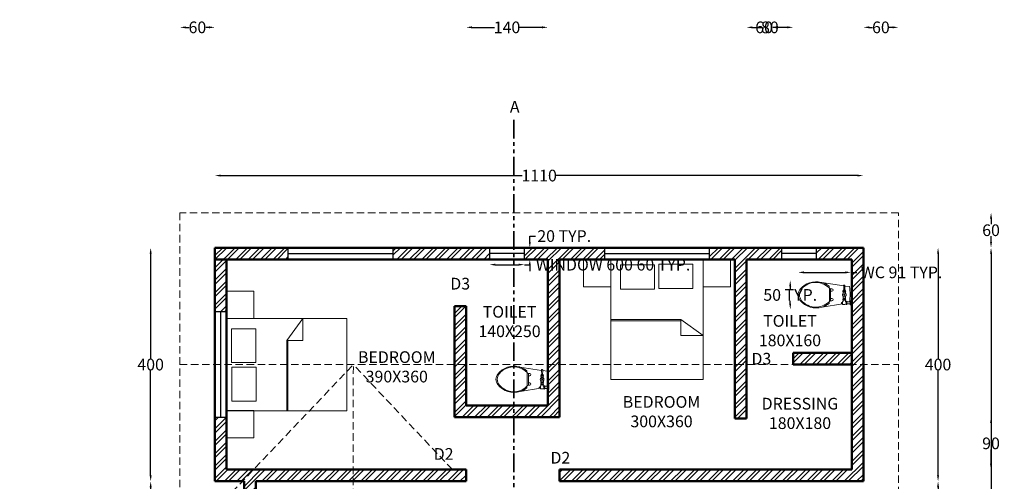
# Model space of a CAD drawing. Units: centimetres. Extents: x 10444 to 13814, y 8288 to 11191.
# Tile 9 of 9: x 12129 to 13814, y 10401 to 11191. Entities that reach past the tile are written whole.
import ezdxf

# ---------------------------------------------------------------- set-up
doc = ezdxf.new("R2010")
doc.units = ezdxf.units.CM
doc.header["$MEASUREMENT"] = 0
doc.linetypes.add('DASHED', pattern=[19.05, 12.7, -6.35])
doc.linetypes.add('PHANTOM', pattern=[63.5, 31.75, -6.35, 6.35, -6.35, 6.35, -6.35])
for name, color, linetype, lineweight in [('A-ANNO-DIMS', 2, 'Continuous', 18), ('A-ANNO-SYMB', 7, 'Continuous', 25), ('A-ANNO-SYMB-SECT', 1, 'PHANTOM', 35), ('A-ANNO-TEXT', 7, 'Continuous', 25), ('A-AREA-IDEN', 3, 'Continuous', 25), ('A-FLOR-FIXT', 9, 'Continuous', 18), ('A-FURN', 8, 'Continuous', 18), ('A-GLAZ', 4, 'Continuous', 25), ('A-ROOF-OVHD', 6, 'DASHED', 18), ('A-WALL', 7, 'Continuous', 50), ('A-WALL-PATT', 8, 'Continuous', 13)]:
    doc.layers.add(name, color=color, linetype=linetype, lineweight=lineweight)
doc.styles.get("Standard").update_dxf_attribs({"font": 'arial.ttf'})
doc.dimstyles.get("Standard").update_dxf_attribs({"dimtxt": 20, "dimasz": 10, "dimexe": 0.18, "dimexo": 0.0625, "dimgap": 0.09, "dimtad": 0, "dimtih": 1, "dimtoh": 1, "dimdec": 0, "dimzin": 0, "dimdsep": 46, "dimtxsty": 'Standard', "dimcen": 0.09, "dimse1": 1, "dimse2": 1, "dimadec": 0, "dimazin": 0, "dimtfac": 1, "dimtdec": 0, "dimtofl": 0, "dimtmove": 0, "dimatfit": 3, "dimfxl": 1, "dimtolj": 1, "dimtzin": 0, "dimarcsym": 0})

# ---------------------------------------------------------------- blocks, each defined once
blk = doc.blocks.new('BED')
for p, q in [((1734.1, 2886.7), (1849.5, 2886.7)), ((1849.5, 2886.7), (1886.1, 2860.2)), ((1886.1, 2860.2), (1849.5, 2886.7)), ((1849.5, 2886.7), (1849.5, 2860.2)), ((1734.1, 2884.7), (1849.5, 2884.7)), ((1849.5, 2860.2), (1886.1, 2860.2))]:
    blk.add_line(p, q)
for points in [[(1734.1, 2787.7), (1886.1, 2787.7), (1886.1, 2985.7), (1734.1, 2985.7)], [(1750, 2936.8), (1805.9, 2936.8), (1805.9, 2977), (1750, 2977)], [(1813.2, 2937.8), (1869.1, 2937.8), (1869.1, 2977.9), (1813.2, 2977.9)]]:
    blk.add_lwpolyline(points, close=True)
blk = doc.blocks.new('TOILETY')
for p, q in [((2296.2, 1053), (2296.2, 1053.3)), ((2296.6, 1052.5), (2297, 1052.5)), ((2297, 1052.5), (2297.7, 1052.5)), ((2297.7, 1052.6), (2297.7, 1052.5)), ((2297.7, 1052.5), (2297.7, 1050.2)), ((2297.7, 1052.5), (2297.7, 1052.5)), ((2303.2, 1052), (2303.2, 1050.7)), ((2307.3, 1052.6), (2307.3, 1052.5)), ((2307.3, 1052.5), (2307.3, 1052.5)), ((2307.3, 1052.5), (2307.3, 1050.2)), ((2297.7, 1050.2), (2297.7, 1050.2)), ((2307.3, 1050.2), (2307.3, 1050.2)), ((2296.5, 1036.2), (2297.2, 1037.4)), ((2297.2, 1037.4), (2297.2, 1038.7)), ((2299.5, 1037.4), (2297.2, 1037.4)), ((2299.5, 1038.7), (2299.5, 1037.4)), ((2303.2, 1037.4), (2299.5, 1037.4)), ((2303.2, 1037.4), (2306.9, 1037.4)), ((2306.9, 1038.7), (2306.9, 1037.4)), ((2306.9, 1037.4), (2309.3, 1037.4)), ((2309.3, 1037.4), (2309.3, 1038.7)), ((2309.9, 1036.2), (2309.3, 1037.4))]:
    blk.add_line(p, q)
for points in [[(2293.8, 1057.3), (2293.3, 1057.3, -0.293225), (2292.6, 1058.4), (2295, 1058.4), (2297.2, 1058.4, -0.293225), (2296.5, 1057.3), (2296, 1057.3)], [(2293.8, 1054.1), (2293.6, 1054.1, 0.913215), (2293.6, 1053.3)], [(2295, 1057.3), (2293.8, 1057.3, -0.293225)], [(2294.9, 1054.1), (2293.8, 1054.1, 0.913215)], [(2294.9, 1054.1), (2296, 1054.1, -0.913215)], [(2295, 1057.3), (2296, 1057.3, 0.335115)], [(2296, 1056.9, -0.066772), (2311.6, 1056.7, -11.173493)], [(2296, 1054.1), (2296.2, 1054.1, -0.913215), (2296.2, 1053.3), (2296.1, 1053.3)], [(2297.8, 1052.7, 0.071269), (2297.8, 1052.5, 0.085783), (2297.9, 1052.4, 0.10607), (2298, 1052.2, 0.126822), (2298.2, 1052.2, 0.126822), (2298.4, 1052.2, 0.10607), (2298.5, 1052.4, 0.085783), (2298.6, 1052.5, 0.071269), (2298.6, 1052.7, 0.075445)], [(2298.7, 1052.6, 0.236068), (2298.8, 1052.5), (2299.8, 1052.5, 0.868488)], [(2306.3, 1052.6, -0.236068), (2306.2, 1052.5), (2304.8, 1052.5, -0.947474)], [(2307.2, 1052.7, -0.071269), (2307.2, 1052.5, -0.085783), (2307.1, 1052.4, -0.10607), (2307, 1052.2, -0.126822), (2306.8, 1052.2, -0.126822), (2306.6, 1052.2, -0.10607), (2306.5, 1052.4, -0.085783), (2306.4, 1052.5, -0.071269), (2306.4, 1052.7, -0.075445)], [(2307.3, 1052.5, 0.414214), (2307.4, 1052.4), (2307.9, 1052.5, -0.274044), (2308, 1052.4), (2308, 1051.9)], [(2308, 1051.9, 0.386607), (2308.3, 1051.8), (2312.2, 1052, -0.016038)], [(2312.2, 1052), (2311.6, 1056.7, 0.064477)], [(2312.2, 1052), (2312.7, 1052, -0.016603), (2312.7, 1052, -1.33807)], [(2312.7, 1052, -0.398884), (2313.2, 1051.6), (2313.2, 1051.4)], [(2312.7, 1050.7, 0.398884), (2313.2, 1051.2), (2313.2, 1051.4)], [(2290.7, 1028.8), (2294, 1049.6, -0.075157)], [(2297.8, 1050.1, -0.056795), (2297.8, 1050.3, -0.085783), (2297.9, 1050.5, -0.10607), (2298, 1050.6, -0.126822), (2298.2, 1050.6, -0.126822), (2298.4, 1050.6, -0.10607), (2298.5, 1050.5, -0.085783), (2298.6, 1050.3, -0.056795), (2298.6, 1050.1, -0.075445)], [(2298.7, 1050.2, -0.236068), (2298.8, 1050.3), (2299.8, 1050.3, -0.868488)], [(2306.3, 1050.2, 0.236068), (2306.2, 1050.3), (2304.8, 1050.3, 0.947474)], [(2307.2, 1050.1, 0.056795), (2307.2, 1050.3, 0.085783), (2307.1, 1050.5, 0.10607), (2307, 1050.6, 0.126822), (2306.8, 1050.6, 0.126822), (2306.6, 1050.6, 0.10607), (2306.5, 1050.5, 0.085783), (2306.4, 1050.3, 0.056795), (2306.4, 1050.1, 0.075445)], [(2307.3, 1050.2, -0.414214), (2307.4, 1050.3), (2307.9, 1050.3, 0.274044), (2308, 1050.3), (2308, 1050.8)], [(2308, 1050.8, -0.386607), (2308.3, 1051), (2312.4, 1050.8, 0.016063)], [(2312.4, 1050.8), (2312.7, 1050.7, 0.016603), (2312.7, 1050.7, 1.33807)], [(2315.8, 1028.5), (2312.4, 1050.8, 0.07524)], [(2296, 1035.7, 0.434217), (2297.2, 1007.6, 0.182634), (2303.2, 1005.4, 2.693815)], [(2294.4, 1035.7, 0.094048), (2290.7, 1028.8, 0.16845)], [(2296, 1035.7), (2294.4, 1035.7, 0.416606)], [(2296.5, 1036.2, 0.008985), (2296, 1035.7, 0.182634)], [(2303.2, 1036.2), (2296.5, 1036.2, 0.008985)], [(2303.2, 1036.2), (2309.9, 1036.2, -0.444938)], [(2310.4, 1035.7, -0.434217), (2309.3, 1007.6, -0.182634), (2303.2, 1005.4, -2.693815)], [(2309.9, 1036.2, -0.008985), (2310.4, 1035.7, -0.182634)], [(2310.4, 1035.7), (2312, 1035.7, -0.416606)], [(2312, 1035.7, -0.105447), (2316, 1027.8, -0.16845)], [(2290.7, 1028.8, 0.310397), (2297.8, 1005.9, 0.16845), (2303.2, 1004, 2.883082)], [(2316, 1027.8, -0.298065), (2308.6, 1005.9, -0.16845), (2303.2, 1004, -2.883082)], [(2316, 1027.8, 0.006132), (2315.8, 1028.5, 0.069947)]]:
    blk.add_lwpolyline(points, format="xyb")
for points in [[(2293.6, 1053.3), (2293.6, 1052.5), (2293.3, 1051.8), (2293.3, 1049.8)], [(2296.2, 1053.3), (2293.6, 1053.3)], [(2293.8, 1054.1), (2293.8, 1057.3)], [(2296, 1056.9), (2296, 1057.3)], [(2296, 1054.1), (2296, 1056.9)], [(2298.7, 1050.2), (2298.7, 1052.6)], [(2299.8, 1052.5), (2299.8, 1052.7), (2301.9, 1052.7)], [(2299.8, 1052.5), (2299.8, 1050.3)], [(2306.3, 1050.2), (2306.3, 1052.6)], [(2308, 1051.9), (2308, 1051.4)], [(2308, 1050.8), (2308, 1051.4)], [(2294, 1049.6), (2293.4, 1049.6), (2293.3, 1049.8)], [(2294.2, 1049.6), (2294, 1049.6)], [(2294.2, 1049.5), (2294.2, 1049.6)], [(2295.4, 1049.6), (2294.2, 1049.6)], [(2294.2, 1049.5), (2294.2, 1049.5)], [(2294.2, 1049.5), (2295.4, 1049.5)], [(2294.3, 1048.9), (2294.2, 1048.9), (2294.2, 1049.5)], [(2294.2, 1049.5), (2294.5, 1049.4), (2294.8, 1049.5), (2295.2, 1049.4), (2295.4, 1049.5)], [(2294.2, 1048.9), (2294.5, 1049), (2294.8, 1048.9), (2295.2, 1049), (2295.4, 1048.9)], [(2294.3, 1048.9), (2294.3, 1048.5), (2294.6, 1048.5)], [(2295.3, 1048.9), (2294.3, 1048.9)], [(2294.5, 1049), (2294.5, 1049.4)], [(2294.6, 1048.5), (2295.3, 1048.5), (2295.3, 1048.9)], [(2295.2, 1049), (2295.2, 1049.4)], [(2295.4, 1049.5), (2295.4, 1049.5), (2295.4, 1048.9), (2295.3, 1048.9)], [(2296.3, 1049.8), (2296.3, 1049.6), (2295.4, 1049.6)], [(2295.4, 1049.5), (2295.4, 1049.6)], [(2296.3, 1049.8), (2296.6, 1050.2)], [(2296.6, 1050.2), (2297.7, 1050.2)], [(2299.8, 1050.3), (2299.8, 1050.1), (2301.8, 1050.1)]]:
    blk.add_lwpolyline(points)
for points in [[(2294.9, 1053.3, 0.06206), (2295.2, 1053.4, 0.075298), (2295.4, 1053.4, 0.107049), (2295.5, 1053.6, 0.150029), (2295.5, 1053.7, 0.150029), (2295.5, 1053.8, 0.107049), (2295.4, 1054, 0.075298), (2295.2, 1054.1, 0.06206), (2294.9, 1054.1, 0.06206), (2294.7, 1054.1, 0.075298), (2294.5, 1054, 0.107049), (2294.3, 1053.8, 0.150029), (2294.3, 1053.7, 0.150029), (2294.3, 1053.6, 0.107049), (2294.5, 1053.4, 0.075298), (2294.7, 1053.4, 0.06206)], [(2298.6, 1051.4, -0.075445), (2298.6, 1051.2, -0.085783), (2298.5, 1051, -0.10607), (2298.4, 1050.8, -0.126822), (2298.2, 1050.8, -0.126822), (2298, 1050.8, -0.10607), (2297.9, 1051, -0.085783), (2297.8, 1051.2, -0.075445), (2297.8, 1051.4, -0.075445), (2297.8, 1051.6, -0.085783), (2297.9, 1051.8, -0.10607), (2298, 1051.9, -0.126822), (2298.2, 1051.9, -0.126822), (2298.4, 1051.9, -0.10607), (2298.5, 1051.8, -0.085783), (2298.6, 1051.6, -0.075445)], [(2306.4, 1051.4, 0.075445), (2306.4, 1051.2, 0.085783), (2306.5, 1051, 0.10607), (2306.6, 1050.8, 0.126822), (2306.8, 1050.8, 0.126822), (2307, 1050.8, 0.10607), (2307.1, 1051, 0.085783), (2307.2, 1051.2, 0.075445), (2307.2, 1051.4, 0.075445), (2307.2, 1051.6, 0.085783), (2307.1, 1051.8, 0.10607), (2307, 1051.9, 0.126822), (2306.8, 1051.9, 0.126822), (2306.6, 1051.9, 0.10607), (2306.5, 1051.8, 0.085783), (2306.4, 1051.6, 0.075445)]]:
    blk.add_lwpolyline(points, format="xyb", close=True)
blk.add_lwpolyline([(2303.2, 1052), (2302.6, 1051.7), (2302.6, 1051), (2303.2, 1050.7), (2303.8, 1051), (2303.8, 1051.7)], close=True)
blk.add_circle((2303.2, 1051.4), 1.91)
for centre, radius, start, end in [((2293.7, 1053.7), 0.391, 275.1944, 84.8056), ((2296.1, 1053.7), 0.391, 95.1944, 264.8056), ((2296.7, 1053), 0.527, 178.4608, 258.8588), ((2298.2, 1052.3), 0.551, 33.3985, 146.6015), ((2306.8, 1052.3), 0.551, 33.3985, 146.6015), ((2298.2, 1050.5), 0.551, 213.3985, 326.6015), ((2306.8, 1050.5), 0.551, 213.3985, 326.6015), ((2298.3, 1038.7), 1.16, 0, 180), ((2308.1, 1038.7), 1.16, 0, 180)]:
    blk.add_arc(centre, radius, start, end)
blk = doc.blocks.new('*D15')
at = {"layer": 'A-ANNO-DIMS', "color": 0, "lineweight": -2, "transparency": 16777216}
for p, q in [((12473.1, 10924.2), (12989.1, 10924.2)), ((13563.1, 10924.2), (13047.1, 10924.2))]:
    blk.add_line(p, q, dxfattribs=at)
at = {"layer": 'A-ANNO-DIMS', "color": 0, "transparency": 16777216}
for points in [[(12473.1, 10925.8), (12473.1, 10922.5), (12463.1, 10924.2)], [(13563.1, 10925.8), (13563.1, 10922.5), (13573.1, 10924.2)]]:
    blk.add_solid(points, dxfattribs=at)
at = {"layer": 'Defpoints', "color": 0, "transparency": 16777216}
for p in [(13573.1, 10924.2), (12463.1, 10800.6), (13573.1, 10800.6)]:
    blk.add_point(p, dxfattribs=at)
at = {"layer": 'A-ANNO-DIMS', "color": 0, "transparency": 16777216, "insert": (13018.1, 10924.2), "char_height": 20, "attachment_point": 5}
blk.add_mtext('\\A1;1110', dxfattribs=at)
blk = doc.blocks.new('*D16')
at = {"layer": 'A-ANNO-DIMS', "color": 0, "lineweight": -2, "transparency": 16777216}
for p, q in [((12353.1, 10790.6), (12353.1, 10610.9)), ((12353.1, 10410.6), (12353.1, 10590.3))]:
    blk.add_line(p, q, dxfattribs=at)
at = {"layer": 'A-ANNO-DIMS', "color": 0, "transparency": 16777216}
for points in [[(12351.5, 10790.6), (12354.8, 10790.6), (12353.1, 10800.6)], [(12351.5, 10410.6), (12354.8, 10410.6), (12353.1, 10400.6)]]:
    blk.add_solid(points, dxfattribs=at)
at = {"layer": 'Defpoints', "color": 0, "transparency": 16777216}
for p in [(12463.1, 10800.6), (12353.1, 10400.6), (12463.1, 10400.6)]:
    blk.add_point(p, dxfattribs=at)
at = {"layer": 'A-ANNO-DIMS', "color": 0, "transparency": 16777216, "insert": (12353.1, 10600.6), "char_height": 20, "attachment_point": 5}
blk.add_mtext('\\A1;400', dxfattribs=at)
blk = doc.blocks.new('*D17')
at = {"layer": 'A-ANNO-DIMS', "color": 0, "lineweight": -2, "transparency": 16777216}
for p, q in [((12353.1, 10390.6), (12353.1, 10170.9)), ((12353.1, 9930.6), (12353.1, 10150.3))]:
    blk.add_line(p, q, dxfattribs=at)
at = {"layer": 'A-ANNO-DIMS', "color": 0, "transparency": 16777216}
for points in [[(12351.5, 10390.6), (12354.8, 10390.6), (12353.1, 10400.6)], [(12351.5, 9930.6), (12354.8, 9930.6), (12353.1, 9920.6)]]:
    blk.add_solid(points, dxfattribs=at)
at = {"layer": 'Defpoints', "color": 0, "transparency": 16777216}
for p in [(12353.1, 10400.6), (12513.1, 10400.6), (12513.1, 9920.6)]:
    blk.add_point(p, dxfattribs=at)
at = {"layer": 'A-ANNO-DIMS', "color": 0, "transparency": 16777216, "insert": (12353.1, 10160.6), "char_height": 20, "attachment_point": 5}
blk.add_mtext('\\A1;480', dxfattribs=at)
blk = doc.blocks.new('*D18')
at = {"layer": 'A-ANNO-DIMS', "color": 0, "lineweight": -2, "transparency": 16777216}
for p, q in [((13700.9, 10790.6), (13700.9, 10610.9)), ((13700.9, 10410.6), (13700.9, 10590.3))]:
    blk.add_line(p, q, dxfattribs=at)
at = {"layer": 'A-ANNO-DIMS', "color": 0, "transparency": 16777216}
for points in [[(13699.3, 10790.6), (13702.6, 10790.6), (13700.9, 10800.6)], [(13699.3, 10410.6), (13702.6, 10410.6), (13700.9, 10400.6)]]:
    blk.add_solid(points, dxfattribs=at)
at = {"layer": 'Defpoints', "color": 0, "transparency": 16777216}
for p in [(13573.1, 10800.6), (13573.1, 10400.6), (13700.9, 10400.6)]:
    blk.add_point(p, dxfattribs=at)
at = {"layer": 'A-ANNO-DIMS', "color": 0, "transparency": 16777216, "insert": (13700.9, 10600.6), "char_height": 20, "attachment_point": 5}
blk.add_mtext('\\A1;400', dxfattribs=at)
blk = doc.blocks.new('*D19')
at = {"layer": 'A-ANNO-DIMS', "color": 0, "lineweight": -2, "transparency": 16777216}
for p, q in [((13700.9, 10390.6), (13700.9, 10170.9)), ((13700.9, 9930.6), (13700.9, 10150.3))]:
    blk.add_line(p, q, dxfattribs=at)
at = {"layer": 'A-ANNO-DIMS', "color": 0, "transparency": 16777216}
for points in [[(13699.3, 10390.6), (13702.6, 10390.6), (13700.9, 10400.6)], [(13699.3, 9930.6), (13702.6, 9930.6), (13700.9, 9920.6)]]:
    blk.add_solid(points, dxfattribs=at)
at = {"layer": 'Defpoints', "color": 0, "transparency": 16777216}
for p in [(13443.1, 10400.6), (13443.1, 9920.6), (13700.9, 9920.6)]:
    blk.add_point(p, dxfattribs=at)
at = {"layer": 'A-ANNO-DIMS', "color": 0, "transparency": 16777216, "insert": (13700.9, 10160.6), "char_height": 20, "attachment_point": 5}
blk.add_mtext('\\A1;480', dxfattribs=at)
blk = doc.blocks.new('WIN-1800')
blk.add_line((0, 10), (180, 10))
blk.add_lwpolyline([(0, 0), (180, 0), (180, 20), (0, 20)], close=True)
blk = doc.blocks.new('WIN-600')
blk.add_line((60, 10), (0, 10))
blk.add_lwpolyline([(0, 0), (60, 0), (60, 20), (0, 20)], close=True)
blk = doc.blocks.new('*D33')
at = {"layer": 'A-ANNO-DIMS', "color": 0, "lineweight": -2, "transparency": 16777216}
for p, q in [((12943.1, 10771.6), (12983.1, 10771.6)), ((12993.1, 10771.6), (13003.1, 10771.6))]:
    blk.add_line(p, q, dxfattribs=at)
at = {"layer": 'A-ANNO-DIMS', "color": 0, "transparency": 16777216}
for points in [[(12943.1, 10773.3), (12943.1, 10770), (12933.1, 10771.6)], [(12983.1, 10773.3), (12983.1, 10770), (12993.1, 10771.6)]]:
    blk.add_solid(points, dxfattribs=at)
at = {"layer": 'Defpoints', "color": 0, "transparency": 16777216}
for p in [(12933.1, 10780.6), (12993.1, 10780.6), (12993.1, 10771.6)]:
    blk.add_point(p, dxfattribs=at)
at = {"layer": 'A-ANNO-DIMS', "color": 0, "transparency": 16777216, "insert": (13144.6, 10771.6), "char_height": 20, "attachment_point": 5}
blk.add_mtext('\\A1;WINDOW 600 60 TYP.', dxfattribs=at)
blk = doc.blocks.new('*D34')
at = {"layer": 'A-ANNO-DIMS', "color": 0, "lineweight": -2, "transparency": 16777216}
for p, q in [((13002.1, 10810.6), (13002.1, 10820.6)), ((13002.1, 10820.6), (13012.1, 10820.6)), ((13002.1, 10770.6), (13002.1, 10760.6))]:
    blk.add_line(p, q, dxfattribs=at)
at = {"layer": 'A-ANNO-DIMS', "color": 0, "transparency": 16777216}
for points in [[(13000.4, 10810.6), (13003.8, 10810.6), (13002.1, 10800.6)], [(13000.4, 10770.6), (13003.8, 10770.6), (13002.1, 10780.6)]]:
    blk.add_solid(points, dxfattribs=at)
at = {"layer": 'Defpoints', "color": 0, "transparency": 16777216}
for p in [(12993.1, 10800.6), (13002.1, 10800.6), (12993.1, 10780.6)]:
    blk.add_point(p, dxfattribs=at)
at = {"layer": 'A-ANNO-DIMS', "color": 0, "transparency": 16777216, "insert": (13061, 10820.6), "char_height": 20, "attachment_point": 5}
blk.add_mtext('\\A1;20 TYP.', dxfattribs=at)
blk = doc.blocks.new('*D37')
at = {"layer": 'A-ANNO-DIMS', "color": 0, "lineweight": -2, "transparency": 16777216}
for p, q in [((13471.5, 10758.4), (13542.1, 10758.4)), ((13552.1, 10758.4), (13562.1, 10758.4))]:
    blk.add_line(p, q, dxfattribs=at)
at = {"layer": 'A-ANNO-DIMS', "color": 0, "transparency": 16777216}
for points in [[(13471.5, 10760.1), (13471.5, 10756.7), (13461.5, 10758.4)], [(13542.1, 10760.1), (13542.1, 10756.7), (13552.1, 10758.4)]]:
    blk.add_solid(points, dxfattribs=at)
at = {"layer": 'Defpoints', "color": 0, "transparency": 16777216}
for p in [(13552.1, 10758.4), (13461.5, 10744.8), (13552.1, 10744.8)]:
    blk.add_point(p, dxfattribs=at)
at = {"layer": 'A-ANNO-DIMS', "color": 0, "transparency": 16777216, "insert": (13638.5, 10758.4), "char_height": 20, "attachment_point": 5}
blk.add_mtext('\\A1;WC 91 TYP.', dxfattribs=at)
blk = doc.blocks.new('*D38')
at = {"layer": 'A-ANNO-DIMS', "color": 0, "lineweight": -2, "transparency": 16777216}
for p, q in [((13447.9, 10734.8), (13447.9, 10730.1)), ((13447.9, 10704.9), (13447.9, 10709.5))]:
    blk.add_line(p, q, dxfattribs=at)
at = {"layer": 'A-ANNO-DIMS', "color": 0, "transparency": 16777216}
for points in [[(13446.2, 10734.8), (13449.5, 10734.8), (13447.9, 10744.8)], [(13446.2, 10704.9), (13449.5, 10704.9), (13447.9, 10694.9)]]:
    blk.add_solid(points, dxfattribs=at)
at = {"layer": 'Defpoints', "color": 0, "transparency": 16777216}
for p in [(13447.9, 10744.8), (13461.5, 10744.8), (13461.5, 10694.9)]:
    blk.add_point(p, dxfattribs=at)
at = {"layer": 'A-ANNO-DIMS', "color": 0, "transparency": 16777216, "insert": (13447.9, 10719.8), "char_height": 20, "attachment_point": 5}
blk.add_mtext('\\A1;50 TYP.', dxfattribs=at)
blk = doc.blocks.new('*D57')
at = {"layer": 'A-ANNO-DIMS', "color": 0, "lineweight": -2, "transparency": 16777216}
for p, q in [((12413.1, 11178), (12418.7, 11178)), ((12453.1, 11178), (12447.5, 11178))]:
    blk.add_line(p, q, dxfattribs=at)
at = {"layer": 'A-ANNO-DIMS', "color": 0, "transparency": 16777216}
for points in [[(12413.1, 11179.7), (12413.1, 11176.3), (12403.1, 11178)], [(12453.1, 11179.7), (12453.1, 11176.3), (12463.1, 11178)]]:
    blk.add_solid(points, dxfattribs=at)
at = {"layer": 'Defpoints', "color": 0, "transparency": 16777216}
for p in [(12463.1, 11178), (12403.1, 10860.6), (12463.1, 10800.6)]:
    blk.add_point(p, dxfattribs=at)
at = {"layer": 'A-ANNO-DIMS', "color": 0, "transparency": 16777216, "insert": (12433.1, 11178), "char_height": 20, "attachment_point": 5}
blk.add_mtext('\\A1;60', dxfattribs=at)
blk = doc.blocks.new('*D58')
at = {"layer": 'A-ANNO-DIMS', "color": 0, "lineweight": -2, "transparency": 16777216}
for p, q in [((13383.1, 11178), (13388.7, 11178)), ((13423.1, 11178), (13417.5, 11178))]:
    blk.add_line(p, q, dxfattribs=at)
at = {"layer": 'A-ANNO-DIMS', "color": 0, "transparency": 16777216}
for points in [[(13383.1, 11179.7), (13383.1, 11176.3), (13373.1, 11178)], [(13423.1, 11179.7), (13423.1, 11176.3), (13433.1, 11178)]]:
    blk.add_solid(points, dxfattribs=at)
at = {"layer": 'Defpoints', "color": 0, "transparency": 16777216}
for p in [(13433.1, 11178), (13433.1, 10800.6), (13373.1, 10780.6)]:
    blk.add_point(p, dxfattribs=at)
at = {"layer": 'A-ANNO-DIMS', "color": 0, "transparency": 16777216, "insert": (13403.1, 11178), "char_height": 20, "attachment_point": 5}
blk.add_mtext('\\A1;60', dxfattribs=at)
blk = doc.blocks.new('*D59')
at = {"layer": 'A-ANNO-DIMS', "color": 0, "lineweight": -2, "transparency": 16777216}
for p, q in [((13583.1, 11178), (13588.7, 11178)), ((13623.1, 11178), (13617.5, 11178))]:
    blk.add_line(p, q, dxfattribs=at)
at = {"layer": 'A-ANNO-DIMS', "color": 0, "transparency": 16777216}
for points in [[(13583.1, 11179.7), (13583.1, 11176.3), (13573.1, 11178)], [(13623.1, 11179.7), (13623.1, 11176.3), (13633.1, 11178)]]:
    blk.add_solid(points, dxfattribs=at)
at = {"layer": 'Defpoints', "color": 0, "transparency": 16777216}
for p in [(13633.1, 11178), (13633.1, 10860.6), (13573.1, 10800.6)]:
    blk.add_point(p, dxfattribs=at)
at = {"layer": 'A-ANNO-DIMS', "color": 0, "transparency": 16777216, "insert": (13603.1, 11178), "char_height": 20, "attachment_point": 5}
blk.add_mtext('\\A1;60', dxfattribs=at)
blk = doc.blocks.new('*D66')
at = {"layer": 'A-ANNO-DIMS', "color": 0, "lineweight": -2, "transparency": 16777216}
for p, q in [((13791.6, 10790.6), (13791.6, 10370.9)), ((13791.6, 9930.6), (13791.6, 10350.3))]:
    blk.add_line(p, q, dxfattribs=at)
at = {"layer": 'A-ANNO-DIMS', "color": 0, "transparency": 16777216}
for points in [[(13789.9, 10790.6), (13793.3, 10790.6), (13791.6, 10800.6)], [(13789.9, 9930.6), (13793.3, 9930.6), (13791.6, 9920.6)]]:
    blk.add_solid(points, dxfattribs=at)
at = {"layer": 'Defpoints', "color": 0, "transparency": 16777216}
for p in [(13573.1, 10800.6), (13443.1, 9920.6), (13791.6, 9920.6)]:
    blk.add_point(p, dxfattribs=at)
at = {"layer": 'A-ANNO-DIMS', "color": 0, "transparency": 16777216, "insert": (13791.6, 10360.6), "char_height": 20, "attachment_point": 5}
blk.add_mtext('\\A1;880', dxfattribs=at)
blk = doc.blocks.new('*D67')
at = {"layer": 'A-ANNO-DIMS', "color": 0, "lineweight": -2, "transparency": 16777216}
for p, q in [((13791.6, 10850.6), (13791.6, 10840.9)), ((13791.6, 10810.6), (13791.6, 10820.3))]:
    blk.add_line(p, q, dxfattribs=at)
at = {"layer": 'A-ANNO-DIMS', "color": 0, "transparency": 16777216}
for points in [[(13789.9, 10850.6), (13793.3, 10850.6), (13791.6, 10860.6)], [(13789.9, 10810.6), (13793.3, 10810.6), (13791.6, 10800.6)]]:
    blk.add_solid(points, dxfattribs=at)
at = {"layer": 'Defpoints', "color": 0, "transparency": 16777216}
for p in [(13633.1, 10860.6), (13791.6, 10860.6), (13573.1, 10800.6)]:
    blk.add_point(p, dxfattribs=at)
at = {"layer": 'A-ANNO-DIMS', "color": 0, "transparency": 16777216, "insert": (13791.6, 10830.6), "char_height": 20, "attachment_point": 5}
blk.add_mtext('\\A1;60', dxfattribs=at)
blk = doc.blocks.new('*D70')
at = {"layer": 'A-ANNO-DIMS', "color": 0, "lineweight": -2, "transparency": 16777216}
for p, q in [((12903.1, 11178), (12941.9, 11178)), ((13023.1, 11178), (12984.3, 11178))]:
    blk.add_line(p, q, dxfattribs=at)
at = {"layer": 'A-ANNO-DIMS', "color": 0, "transparency": 16777216}
for points in [[(12903.1, 11179.7), (12903.1, 11176.3), (12893.1, 11178)], [(13023.1, 11179.7), (13023.1, 11176.3), (13033.1, 11178)]]:
    blk.add_solid(points, dxfattribs=at)
at = {"layer": 'Defpoints', "color": 0, "transparency": 16777216}
for p in [(13033.1, 11178), (13033.1, 10780.6), (12893.1, 10700.6)]:
    blk.add_point(p, dxfattribs=at)
at = {"layer": 'A-ANNO-DIMS', "color": 0, "transparency": 16777216, "insert": (12963.1, 11178), "char_height": 20, "attachment_point": 5}
blk.add_mtext('\\A1;140', dxfattribs=at)
blk = doc.blocks.new('*D86')
at = {"layer": 'A-ANNO-DIMS', "color": 0, "lineweight": -2, "transparency": 16777216}
for p, q in [((13383.1, 11178), (13398.7, 11178)), ((13443.1, 11178), (13427.5, 11178))]:
    blk.add_line(p, q, dxfattribs=at)
at = {"layer": 'A-ANNO-DIMS', "color": 0, "transparency": 16777216}
for points in [[(13383.1, 11179.7), (13383.1, 11176.3), (13373.1, 11178)], [(13443.1, 11179.7), (13443.1, 11176.3), (13453.1, 11178)]]:
    blk.add_solid(points, dxfattribs=at)
at = {"layer": 'Defpoints', "color": 0, "transparency": 16777216}
for p in [(13453.1, 11178), (13373.1, 10600.6), (13453.1, 10600.6)]:
    blk.add_point(p, dxfattribs=at)
at = {"layer": 'A-ANNO-DIMS', "color": 0, "transparency": 16777216, "insert": (13413.1, 11178), "char_height": 20, "attachment_point": 5}
blk.add_mtext('\\A1;80', dxfattribs=at)
blk = doc.blocks.new('*D87')
at = {"layer": 'A-ANNO-DIMS', "color": 0, "lineweight": -2, "transparency": 16777216}
for p, q in [((13791.6, 10500.6), (13791.6, 10475.9)), ((13791.6, 10430.6), (13791.6, 10455.3))]:
    blk.add_line(p, q, dxfattribs=at)
at = {"layer": 'A-ANNO-DIMS', "color": 0, "transparency": 16777216}
for points in [[(13789.9, 10500.6), (13793.3, 10500.6), (13791.6, 10510.6)], [(13789.9, 10430.6), (13793.3, 10430.6), (13791.6, 10420.6)]]:
    blk.add_solid(points, dxfattribs=at)
at = {"layer": 'Defpoints', "color": 0, "transparency": 16777216}
for p in [(13053.1, 10510.6), (13791.6, 10510.6), (13053.1, 10420.6)]:
    blk.add_point(p, dxfattribs=at)
at = {"layer": 'A-ANNO-DIMS', "color": 0, "transparency": 16777216, "insert": (13791.6, 10465.6), "char_height": 20, "attachment_point": 5}
blk.add_mtext('\\A1;90', dxfattribs=at)

msp = doc.modelspace()

# ---------------------------------------------------------------- hatches: boundary and pattern name
at = {"layer": 'A-WALL-PATT'}
h = msp.add_hatch(dxfattribs=at)
h.set_pattern_fill('ANSI32', color=256, scale=40)
h.paths.add_polyline_path([(12933.1062, 10800.6336), (12768.1062, 10800.6336), (12768.1062, 10780.6336), (12933.1062, 10780.6336)])
h.paths.add_polyline_path([(12588.1062, 10800.6336), (12463.1062, 10800.6336), (12463.1062, 10780.6336), (12588.1062, 10780.6336)])
h.paths.add_polyline_path([(12483.1062, 10726.41), (12483.1062, 10780.6336), (12463.1062, 10780.6336), (12463.1062, 10690.6336), (12483.1062, 10690.6336)])
h.paths.add_polyline_path([(12483.1062, 10510.6336), (12463.1062, 10510.6336), (12463.1062, 10400.6336), (12510.094, 10400.6336), (12529.0899, 10420.6336), (12483.1062, 10420.6336)])
h.paths.add_polyline_path([(12699.6814, 10420.6336), (12529.0899, 10420.6336), (12510.094, 10400.6336), (12513.1062, 10400.6336), (12513.1062, 10340.6336), (12533.1062, 10340.6336), (12533.1062, 10400.6336), (12699.64, 10400.6336)])
h.paths.add_polyline_path([(12893.1062, 10420.6336), (12699.6814, 10420.6336), (12699.64, 10400.6336), (12893.1062, 10400.6336)])
h.paths.add_polyline_path([(13129.7438, 10800.6336), (12993.1062, 10800.6336), (12993.1062, 10780.6336), (13033.1062, 10780.6336), (13033.1062, 10600.6336), (13053.1062, 10600.6336), (13053.1062, 10780.6336), (13129.7438, 10780.6336)])
h.paths.add_polyline_path([(13433.1062, 10800.6336), (13309.7438, 10800.6336), (13309.7438, 10780.6336), (13345.5201, 10780.6336), (13353.1062, 10780.6336), (13353.1062, 10600.6336), (13373.1062, 10600.6336), (13373.1062, 10780.6336), (13433.1062, 10780.6336)])
h.paths.add_polyline_path([(13573.1062, 10800.6336), (13493.1062, 10800.6336), (13493.1062, 10780.6336), (13553.1062, 10780.6336), (13553.1062, 10600.6336), (13573.1062, 10600.6336)])
h.paths.add_polyline_path([(13573.1062, 10600.6336), (13553.1062, 10600.6336), (13553.1062, 10420.6336), (13053.1062, 10420.6336), (13053.1062, 10400.6336), (13573.1062, 10400.6336)])
h.paths.add_polyline_path([(13053.1062, 10300.6336), (13033.1062, 10300.6336), (13033.1062, 9940.6336), (13013.1062, 9940.6336), (13013.1062, 9920.6336), (13053.1062, 9920.6336)])
h.paths.add_polyline_path([(12993.1062, 9940.6336), (12975, 9940.6336), (12975, 9920.6336), (12993.1062, 9920.6336)])
h.paths.add_polyline_path([(12953.1062, 9940.6336), (12933.1062, 9940.6336), (12933.1062, 9920.6336), (12953.1062, 9920.6336)])
h.paths.add_polyline_path([(12913.1062, 9940.6336), (12893.1062, 9940.6336), (12893.1062, 9920.6336), (12913.1062, 9920.6336)])
h.paths.add_polyline_path([(12873.1062, 9940.6336), (12853.1062, 9940.6336), (12853.1062, 10300.6336), (12833.1062, 10300.6336), (12833.1062, 9920.6336), (12873.1062, 9920.6336)])
h.paths.add_polyline_path([(12733.1062, 10100.6336), (12699.0201, 10100.6336), (12698.9788, 10080.6336), (12733.1062, 10080.6336)])
h.paths.add_polyline_path([(12699.0201, 10100.6336), (12653.1062, 10100.6336), (12653.1062, 10080.6336), (12698.9788, 10080.6336)])
h.paths.add_polyline_path([(12593.1062, 10100.6336), (12533.1062, 10100.6336), (12533.1062, 10160.6336), (12513.1062, 10160.6336), (12513.1062, 10080.6336), (12593.1062, 10080.6336)])
h.paths.add_polyline_path([(13053.1062, 10600.6336), (13033.1062, 10600.6336), (13033.1062, 10576.2537, -0.004993085), (13033.1062, 10574.2995), (13033.1062, 10564.3331, -0.269473124), (13034.9053, 10565.2433), (13034.9053, 10561.5839), (13034.9053, 10557.6884, -0.269473124), (13033.1062, 10558.5987), (13033.1062, 10530.6336), (12975, 10530.6336), (12975, 10510.6336), (13053.1062, 10510.6336)])
h.paths.add_polyline_path([(12975, 10530.6336), (12893.1062, 10530.6336), (12893.1062, 10600.6336), (12873.1062, 10600.6336), (12873.1062, 10510.6336), (12975, 10510.6336)])
h.paths.add_polyline_path([(12893.1062, 10700.6336), (12873.1062, 10700.6336), (12873.1062, 10600.6336), (12893.1062, 10600.6336)])
h.paths.add_polyline_path([(13373.1062, 10600.6336), (13353.1062, 10600.6336), (13353.1062, 10507.9506), (13373.1062, 10507.9506)], flags=17)
h.paths.add_polyline_path([(13553.1062, 10620.6336), (13453.1062, 10620.6336), (13453.1062, 10600.6336), (13553.1062, 10600.6336)])
h.paths.add_polyline_path([(11114.7881, 10700.6336), (11094.7881, 10700.6336), (11094.7881, 10510.6336), (11196.6819, 10510.6336), (11196.6819, 10530.6336), (11114.7881, 10530.6336)])

# ---------------------------------------------------------------- linework, layer by layer
at = {"layer": 'A-ANNO-SYMB-SECT'}
msp.add_line((12975, 11019.5), (12975, 9676.5), dxfattribs=at)
at = {"layer": 'A-FURN'}
for points in [[(13140.7438, 10780.6336), (13093.9675, 10780.6336), (13093.9675, 10733.8573), (13140.7438, 10733.8573)], [(13345.5201, 10780.6336), (13298.7438, 10780.6336), (13298.7438, 10733.8573), (13345.5201, 10733.8573)], [(12483.1062, 10726.41), (12483.1062, 10679.6336), (12529.8825, 10679.6336), (12529.8825, 10726.41)], [(12483.1062, 10521.6336), (12483.1062, 10474.8573), (12529.8825, 10474.8573), (12529.8825, 10521.6336)]]:
    msp.add_lwpolyline(points, close=True, dxfattribs=at)
at = {"layer": 'A-ROOF-OVHD'}
for p, q in [((12403.1062, 10860.6336), (12403.1062, 10340.6336)), ((13633.1062, 10860.6336), (12403.1062, 10860.6336)), ((13633.1062, 10340.6336), (13633.1062, 10860.6336)), ((12403.1062, 10600.6336), (13453.1062, 10600.6336)), ((12453.1062, 10340.6336), (12700.0533, 10600.6336)), ((12698.5242, 9860.6336), (12700.0533, 10600.6336)), ((12869.6073, 10420.6336), (12700.0533, 10600.6336)), ((13453.1062, 10600.6336), (13633.1062, 10600.6336))]:
    msp.add_line(p, q, dxfattribs=at)
at = {"layer": 'A-WALL'}
for p, q in [((13573.1062, 10800.6336), (12463.1062, 10800.6336)), ((12463.1062, 10800.6336), (12463.1062, 10400.6336)), ((13573.1062, 10400.6336), (13573.1062, 10800.6336)), ((13033.1062, 10780.6336), (12463.1062, 10780.6336)), ((12483.1062, 10780.6336), (12893.1062, 10780.6336)), ((12483.1062, 10780.6336), (12483.1062, 10420.6336)), ((12893.1062, 10780.6336), (13033.1062, 10780.6336)), ((13033.1062, 10780.6336), (13033.1062, 10530.6336)), ((13053.1062, 10780.6336), (13053.1062, 10510.6336)), ((13353.1062, 10780.6336), (13053.1062, 10780.6336)), ((13353.1062, 10507.9506), (13353.1062, 10780.6336)), ((13553.1062, 10780.6336), (13373.1062, 10780.6336)), ((13373.1062, 10507.9506), (13373.1062, 10780.6336)), ((13553.1062, 10420.6336), (13553.1062, 10780.6336)), ((12873.1062, 10700.6336), (12873.1062, 10510.6336)), ((12893.1062, 10700.6336), (12873.1062, 10700.6336)), ((12893.1062, 10700.6336), (12893.1062, 10530.6336)), ((13374.8333, 10620.6336), (13373.1062, 10620.6336)), ((13553.1062, 10620.6336), (13453.1062, 10620.6336)), ((13453.1062, 10600.6336), (13453.1062, 10620.6336)), ((13374.8333, 10600.6336), (13373.1062, 10600.6336)), ((13553.1062, 10600.6336), (13453.1062, 10600.6336)), ((12893.1062, 10530.6336), (13033.1062, 10530.6336)), ((12873.1062, 10510.6336), (13053.1062, 10510.6336)), ((13353.1062, 10507.9506), (13373.1062, 10507.9506)), ((12483.1062, 10420.6336), (12893.1062, 10420.6336)), ((12893.1062, 10420.6336), (12893.1062, 10400.6336)), ((13553.1062, 10420.6336), (13053.1062, 10420.6336)), ((13053.1062, 10420.6336), (13053.1062, 10400.6336)), ((12463.1062, 10400.6336), (12513.1062, 10400.6336)), ((12513.1062, 10400.6336), (12513.1062, 9920.6336)), ((12533.1062, 10400.6336), (12893.1062, 10400.6336)), ((12533.1062, 10400.6336), (12533.1062, 10100.6336)), ((13053.1062, 10400.6336), (13573.1062, 10400.6336))]:
    msp.add_line(p, q, dxfattribs=at)

# ---------------------------------------------------------------- block references
at = {"layer": 'A-FLOR-FIXT', "xscale": -1.667297040358401, "yscale": 1.667297040358401, "zscale": 1.667297040358401, "rotation": 270}
for p in [(11787.4284, 6879.8514), (11270.2073, 6735.1716)]:
    msp.add_blockref('TOILETY', p, dxfattribs=at)
at = {"layer": 'A-FURN', "xscale": 1.039473684210526, "yscale": 1.039473684210526, "zscale": 1.039473684210526}
msp.add_blockref('BED', (11338.1512, 7677.0366), dxfattribs=at)
at = {"layer": 'A-FURN', "xscale": 1.039473684210526, "yscale": 1.039473684210526, "zscale": 1.039473684210526, "rotation": 89.99999999999999}
msp.add_blockref('BED', (15586.7032, 8719.0411), dxfattribs=at)
at = {"layer": 'A-GLAZ'}
for name, p in [('WIN-1800', (12588.1061, 10780.634)), ('WIN-600', (12933.1061, 10780.634)), ('WIN-1800', (13129.7437, 10780.634)), ('WIN-600', (13433.1061, 10780.634))]:
    msp.add_blockref(name, p, dxfattribs=at)
at = {"layer": 'A-GLAZ', "rotation": 89.99999999999767}
msp.add_blockref('WIN-1800', (12483.1058, 10510.6335), dxfattribs=at)

# ---------------------------------------------------------------- texts
at = {"layer": 'A-ANNO-SYMB', "insert": (12968, 11052), "char_height": 20, "attachment_point": 1}
msp.add_mtext_dynamic_manual_height_columns('A', width=668.5, gutter_width=1, heights=[0], dxfattribs=at)
at = {"layer": 'A-ANNO-TEXT', "char_height": 20, "attachment_point": 1}
for s, insert in [('D3', (12866, 10749.0819)), ('D3', (13381.5, 10620.5819)), ('D2', (12837.6773, 10457.4966)), ('D2', (13037.5, 10450.9966))]:
    msp.add_mtext_dynamic_manual_height_columns(s, width=668.5, gutter_width=1, heights=[0], dxfattribs=dict(at, insert=insert))
at = {"layer": 'A-AREA-IDEN', "char_height": 20, "attachment_point": 1}
for s, insert in [('\\pxqc;TOILET\\P140X250', (12893.1062, 10700.9016)), ('\\pxqc;TOILET\\P180X160', (13373.1062, 10685.2992)), ('\\pxqc;BEDROOM\\P390X360', (12700.0533, 10623.315)), ('\\pxqc;BEDROOM\\P300X360', (13153.2621, 10546.5772)), ('\\pxqc;DRESSING\\P180X180', (13390.2948, 10543.5988))]:
    msp.add_mtext_dynamic_manual_height_columns(s, width=148.64167, gutter_width=1, heights=[0], dxfattribs=dict(at, insert=insert))

# ---------------------------------------------------------------- dimensions: what is measured, and where the dimension line sits
at = {"layer": 'A-ANNO-DIMS'}
for base, p1, p2, picture, middle in [((12463.1062, 11178), (12403.1062, 10860.6336), (12463.1062, 10800.6336), '*D57', (12433.1062, 11178)), ((13033.1062, 11178), (12893.1062, 10700.6336), (13033.1062, 10780.6336), '*D70', (12963.1062, 11178)), ((13433.1062, 11178), (13373.1062, 10780.6336), (13433.1062, 10800.6336), '*D58', (13403.1062, 11178)), ((13453.1062, 11178), (13373.1062, 10600.6336), (13453.1062, 10600.6336), '*D86', (13413.1062, 11178)), ((13633.1062, 11178), (13573.1062, 10800.6336), (13633.1062, 10860.6336), '*D59', (13603.1062, 11178))]:
    dim = msp.add_linear_dim(base=base, p1=p1, p2=p2, dimstyle='Standard', override={"dimdec": 0, "dimlfac": 1, "dimrnd": 0, "dimzin": 0, "dimdsep": 46, "dimlunit": 2}, dxfattribs=at)
    dim.commit()
    dim.dimension.update_dxf_attribs({"geometry": picture, "text_midpoint": middle})
for p1, p2, distance, picture, middle in [((12463.1062, 10800.6336), (13573.1062, 10800.6336), 123.5274, '*D15', (13018.1062, 10924.1611)), ((12463.1062, 10800.6336), (12463.1062, 10400.6336), -109.9671, '*D16', (12353.1391, 10600.6336)), ((13573.1062, 10800.6336), (13573.1062, 10400.6336), 127.8354, '*D18', (13700.9416, 10600.6336)), ((12513.1062, 9920.6336), (12513.1062, 10400.6336), 159.9671, '*D17', (12353.1391, 10160.6336)), ((13443.1062, 10400.6336), (13443.1062, 9920.6336), 257.8354, '*D19', (13700.9416, 10160.6336))]:
    dim = msp.add_aligned_dim(p1=p1, p2=p2, distance=distance, dimstyle='Standard', override={"dimclrd": 0, "dimclre": 0, "dimclrt": 0}, dxfattribs=at)
    dim.commit()
    dim.dimension.update_dxf_attribs({"geometry": picture, "text_midpoint": middle})
for base, p1, p2, picture, middle in [((13791.6062, 10860.6336), (13573.1062, 10800.6336), (13633.1062, 10860.6336), '*D67', (13791.6062, 10830.6336)), ((13791.6062, 9920.6336), (13573.1062, 10800.6336), (13443.1062, 9920.6336), '*D66', (13791.6062, 10360.6336)), ((13791.6062, 10510.6336), (13053.1062, 10420.6336), (13053.1062, 10510.6336), '*D87', (13791.6062, 10465.6336))]:
    dim = msp.add_linear_dim(base=base, p1=p1, p2=p2, angle=90, dimstyle='Standard', override={"dimdec": 0, "dimlfac": 1, "dimrnd": 0, "dimzin": 0, "dimdsep": 46, "dimlunit": 2}, dxfattribs=at)
    dim.commit()
    dim.dimension.update_dxf_attribs({"geometry": picture, "text_midpoint": middle})
for base, p1, p2, picture, middle in [((13002.1062, 10800.6336), (12993.1062, 10780.6336), (12993.1062, 10800.6336), '*D34', (13061.0434, 10820.6336)), ((13447.863, 10744.7916), (13461.4625, 10694.8613), (13461.4625, 10744.7916), '*D38', (13447.863, 10719.8264))]:
    dim = msp.add_linear_dim(base=base, p1=p1, p2=p2, angle=90, text='<> TYP.', dimstyle='Standard', override={"dimdec": 0, "dimrnd": 0, "dimzin": 0, "dimlunit": 2}, dxfattribs=at)
    dim.commit()
    dim.dimension.update_dxf_attribs({"geometry": picture, "text_midpoint": middle})
for base, p1, p2, text, picture, middle in [((12993.1062, 10771.6336), (12933.1062, 10780.6336), (12993.1062, 10780.6336), 'WINDOW 600 <> TYP.', '*D33', (13144.6491, 10771.6336)), ((13552.1264, 10758.3912), (13461.4625, 10744.7916), (13552.1264, 10744.7916), 'WC <> TYP.', '*D37', (13638.4579, 10758.3912))]:
    dim = msp.add_linear_dim(base=base, p1=p1, p2=p2, text=text, dimstyle='Standard', override={"dimdec": 0, "dimrnd": 0, "dimzin": 0, "dimlunit": 2}, dxfattribs=at)
    dim.commit()
    dim.dimension.update_dxf_attribs({"geometry": picture, "text_midpoint": middle})

doc.saveas('drawing.dxf')
